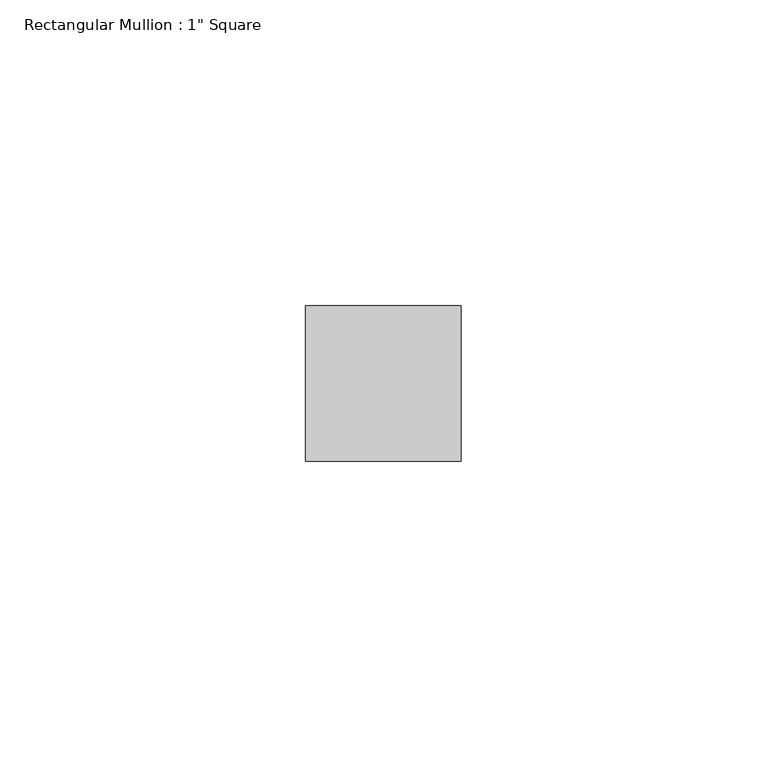
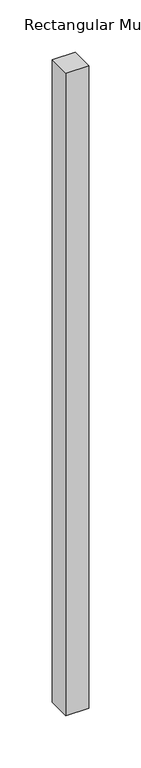
"""IFC4 building model written with IfcOpenShell, lengths in millimetres: member geometry."""

from ifc_helpers import new_model, si_unit, frame, origin, place, context, project, spatial, polyline, outline, extrude, source, transform, mapped, element, save


def member_12606fcf(model_context):
    return source(origin(), model_context, "Body", "SweptSolid", [
        extrude(outline(polyline([(12.7, 12.7), (12.7, -12.7), (-12.7, -12.7), (-12.7, 12.7), (12.7, 12.7)])), frame((0.0, 0.0, -749.3), z_axis=(0.0, 0.0, 1.0), x_axis=(1.0, 0.0, 0.0)), (0.0, 0.0, 1.0), 749.3),
    ])


if __name__ == "__main__":
    model = new_model("IFC4")
    model_context = context("Model", 3, world=origin())
    ifc_project = project(units=[si_unit("LENGTHUNIT", "METRE", prefix="MILLI")], contexts=[model_context])
    site = spatial("IfcSite", under=ifc_project)
    building = spatial("IfcBuilding", under=site)
    placement = place(None, origin())
    member_shape = member_12606fcf(model_context)
    element("IfcMember", 1, ObjectType="Rectangular Mullion : 1\" Square", at=placement, inside=building, context=model_context, shape_type="MappedRepresentation", body=[
        mapped(member_shape, transform((0.0, 0.0, 0.0), x_axis=(1.0, 0.0, 0.0), y_axis=(0.0, 1.0, 0.0), z_axis=(0.0, 0.0, 1.0))),
    ])
    save(model, "model.ifc")

# Revit data of these elements
# Type "Rectangular Mullion : 1\" Square"
#   built-in parameter 1007304 = 0.0833333 (stored number, unit not read)
#   built-in parameter 1007301 = 0.0416667 (stored number, unit not read)
#   built-in parameter 1007300 = 0.0416667 (stored number, unit not read)
# Element 1 (IfcMember, "Rectangular Mullion : 1\" Square")
#   Materials on its faces: "Aluminum"
# Materials
#   "Aluminum": class "Metal", colour RGB 247 247 247, transparency 0, Description = "Aluminum 6061", Cost = 0
